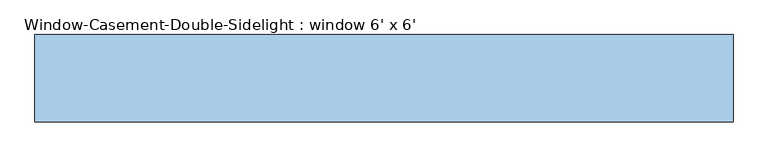
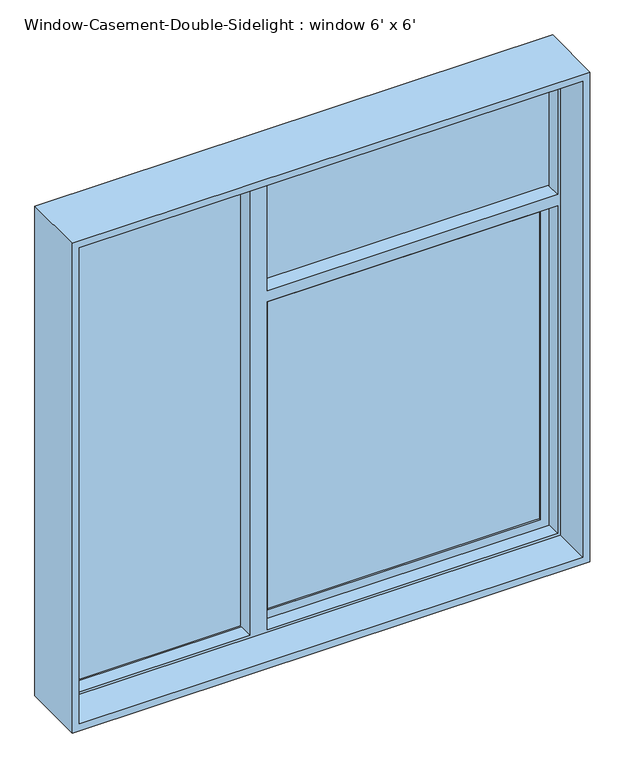
"""IFC4 building model written with IfcOpenShell, lengths in millimetres: window geometry, Window-Casement-Double-Sidelight : window 6' x 6'."""

from ifc_helpers import new_model, si_unit, frame, origin, place, context, project, spatial, polyline, outline, extrude, faceted_brep, source, transform, mapped, element, save


def window_casement_double_sidelight_window_6_x_6_6a7c62ef(model_context):
    return source(origin(), model_context, "Body", "SolidModel", [
        extrude(outline(polyline([(847.1296875, 98.425), (-115.6096875, 98.425), (-115.6096875, 111.125), (847.1296875, 111.125), (847.1296875, 98.425)])), frame((0.0, 0.0, 981.6703125), z_axis=(0.0, 0.0, 1.0), x_axis=(1.0, 0.0, 0.0)), (0.0, 0.0, 1.0), 1150.0842187),
        extrude(outline(polyline([(847.1296875, 85.725), (847.1296875, 79.375), (-115.6096875, 79.375), (-115.6096875, 85.725), (847.1296875, 85.725)])), frame((0.0, 0.0, 981.6703125), z_axis=(0.0, 0.0, 1.0), x_axis=(1.0, 0.0, 0.0)), (0.0, 0.0, 1.0), 1150.0842187),
        extrude(outline(polyline([(-208.28, 98.425), (-208.28, 92.075), (-889.0, 92.075), (-889.0, 98.425), (-208.28, 98.425)])), frame((0.0, 0.0, 949.9203125), z_axis=(0.0, 0.0, 1.0), x_axis=(1.0, 0.0, 0.0)), (0.0, 0.0, 1.0), 1767.8796875),
        extrude(outline(polyline([(-208.28, 85.725), (-208.28, 79.375), (-889.0, 79.375), (-889.0, 85.725), (-208.28, 85.725)])), frame((0.0, 0.0, 949.9203125), z_axis=(0.0, 0.0, 1.0), x_axis=(1.0, 0.0, 0.0)), (0.0, 0.0, 1.0), 1767.8796875),
        extrude(outline(polyline([(889.0, 85.725), (889.0, 79.375), (-157.48, 79.375), (-157.48, 85.725), (889.0, 85.725)])), frame((0.0, 0.0, 2215.4951563), z_axis=(0.0, 0.0, 1.0), x_axis=(1.0, 0.0, 0.0)), (0.0, 0.0, 1.0), 502.3048438),
        extrude(outline(polyline([(889.0, 98.425), (889.0, 92.075), (-157.48, 92.075), (-157.48, 98.425), (889.0, 98.425)])), frame((0.0, 0.0, 2215.4951563), z_axis=(0.0, 0.0, 1.0), x_axis=(1.0, 0.0, 0.0)), (0.0, 0.0, 1.0), 502.3048438),
        faceted_brep([(-889.0, 73.025, 2717.8), (-889.0, 114.3, 2717.8), (889.0, 114.3, 2717.8), (889.0, 73.025, 2717.8), (-157.48, 73.025, 2717.8), (-157.48, 111.125, 2717.8), (-208.28, 111.125, 2717.8), (-208.28, 73.025, 2717.8), (-878.8796875, 22.225, 2707.6796875), (-878.8796875, 73.025, 2707.6796875), (-208.28, 73.025, 2707.6796875), (-208.28, 22.225, 2707.6796875), (878.8796875, 73.025, 2707.6796875), (878.8796875, 22.225, 2707.6796875), (-147.3596875, 22.225, 2707.6796875), (-147.3596875, 73.025, 2707.6796875), (-889.0, -114.3, 2717.8), (-889.0, 22.225, 2717.8), (889.0, 22.225, 2717.8), (889.0, -114.3, 2717.8), (-914.4, 114.3, 2743.2), (-914.4, -114.3, 2743.2), (914.4, -114.3, 2743.2), (914.4, 114.3, 2743.2), (889.0, 114.3, 939.8), (889.0, 73.025, 939.8), (889.0, 73.025, 2173.6248438), (889.0, 111.125, 2173.6248438), (889.0, 111.125, 2215.4951563), (889.0, 73.025, 2215.4951563), (878.8796875, 73.025, 2215.4951563), (878.8796875, 22.225, 2215.4951563), (878.8796875, 73.025, 949.9203125), (878.8796875, 22.225, 949.9203125), (878.8796875, 22.225, 2173.6248438), (878.8796875, 73.025, 2173.6248438), (889.0, 22.225, 939.8), (889.0, -114.3, 939.8), (914.4, -114.3, 914.4), (914.4, 114.3, 914.4), (-889.0, 114.3, 939.8), (-889.0, 73.025, 939.8), (-208.28, 73.025, 939.8), (-208.28, 111.125, 939.8), (-157.48, 111.125, 939.8), (-157.48, 73.025, 939.8), (-147.3596875, 73.025, 949.9203125), (-147.3596875, 22.225, 949.9203125), (-878.8796875, 73.025, 949.9203125), (-878.8796875, 22.225, 949.9203125), (-208.28, 22.225, 949.9203125), (-208.28, 73.025, 949.9203125), (-889.0, 22.225, 939.8), (-889.0, -114.3, 939.8), (-914.4, -114.3, 914.4), (-914.4, 114.3, 914.4), (-147.3596875, 73.025, 2215.4951563), (-157.48, 73.025, 2215.4951563), (-157.48, 73.025, 2173.6248438), (-147.3596875, 73.025, 2173.6248438), (-147.3596875, 22.225, 2215.4951563), (-147.3596875, 22.225, 2173.6248438), (-157.48, 111.125, 2215.4951563), (-157.48, 111.125, 2173.6248438)], [[[0, 1, 2, 3, 4, 5, 6, 7]], [[8, 9, 10, 11]], [[12, 13, 14, 15]], [[16, 17, 18, 19]], [[20, 21, 22, 23]], [[3, 2, 24, 25, 26, 27, 28, 29]], [[13, 12, 30, 31]], [[32, 33, 34, 35]], [[19, 18, 36, 37]], [[23, 22, 38, 39]], [[25, 24, 40, 41, 42, 43, 44, 45]], [[33, 32, 46, 47]], [[48, 49, 50, 51]], [[37, 36, 52, 53]], [[39, 38, 54, 55]], [[1, 0, 41, 40]], [[12, 15, 56, 57, 4, 3, 29, 30]], [[46, 32, 35, 26, 25, 45, 58, 59]], [[41, 0, 7, 10, 9, 48, 51, 42]], [[9, 8, 49, 48]], [[17, 52, 36, 18], [13, 31, 60, 14], [33, 47, 61, 34], [49, 8, 11, 50]], [[17, 16, 53, 52]], [[22, 21, 54, 38], [16, 19, 37, 53]], [[21, 20, 55, 54]], [[20, 23, 39, 55], [2, 1, 40, 24]], [[43, 6, 5, 62, 28, 27, 63, 44]], [[6, 43, 42, 51, 50, 11, 10, 7]], [[15, 14, 60, 56]], [[47, 46, 59, 61]], [[5, 4, 57, 62]], [[45, 44, 63, 58]], [[63, 27, 26, 35, 34, 61, 59, 58]], [[28, 62, 57, 56, 60, 31, 30, 29]]]),
        extrude(outline(polyline([(2173.6248438, 889.0), (2173.6248438, -157.48), (939.8, -157.48), (939.8, 889.0), (2173.6248438, 889.0)]), holes=[polyline([(981.6703125, 847.1296875), (981.6703125, -115.6096875), (2131.7545313, -115.6096875), (2131.7545313, 847.1296875), (981.6703125, 847.1296875)])]), frame((0.0, 73.025, 0.0), z_axis=(0.0, 1.0, 0.0), x_axis=(0.0, 0.0, 1.0)), (0.0, 0.0, 1.0), 31.75),
    ])


if __name__ == "__main__":
    model = new_model("IFC4")
    model_context = context("Model", 3, world=origin())
    ifc_project = project(units=[si_unit("LENGTHUNIT", "METRE", prefix="MILLI")], contexts=[model_context])
    site = spatial("IfcSite", under=ifc_project)
    building = spatial("IfcBuilding", under=site)
    placement = place(None, origin())
    window_casement_double_sidelight_window_6_x_6_shape = window_casement_double_sidelight_window_6_x_6_6a7c62ef(model_context)
    element("IfcWindow", 1, ObjectType="Window-Casement-Double-Sidelight : window 6' x 6'", at=placement, inside=building, context=model_context, shape_type="MappedRepresentation", body=[
        mapped(window_casement_double_sidelight_window_6_x_6_shape, transform((0.0, 0.0, 0.0), x_axis=(1.0, 0.0, 0.0), y_axis=(0.0, 1.0, 0.0), z_axis=(0.0, 0.0, 1.0))),
    ])
    save(model, "model.ifc")

# Revit data of these elements
# Type "Window-Casement-Double-Sidelight : window 6' x 6'"
#   Type Mark = "23"
#   Fire Rating = "0.5h"
#   Assembly Code = "B2020100"
#   Analytic Construction = "Double glazing - domestic"
#   Window Inset [instance default] = 0' - 0 5/8"
#   Wall Thickness [instance default] = 0' - 6"
#   Visual Light Transmittance = 0.81
#   Transom Height Ratio = 0.3
#   Transom Height = 1' - 9.6"
#   Thermal Resistance (R) = 1.8146 (h·ft²·°F)/BTU
#   Solar Heat Gain Coefficient = 0.76
#   Side Width = 2' - 4.8"
#   Rough Width = 6' - 0 1/2"
#   Rough Height = 6' - 0 1/2"
#   Opening Window Width = 3' - 7.2"
#   Opening Window Height = 4' - 2.4"
#   Heat Transfer Coefficient (U) = 0.5511 BTU/(h·ft²·°F)
#   Height = 6' - 0"
#   Frame Gap 3 [instance default] = 0' - 1 83/128"
#   Frame Gap 2 [instance default] = 0' - 0 5/8"
#   Frame Gap 1 = 0' - 1 51/128"
#   Default Sill Height = 3' - 0"
#   Width = 6' - 0"
#   Frame Material = Metal - Aluminum
#   Glass Panel Material = Glass
#   Wall Closure = (empty or 0)
# Element 1 (IfcWindow, "Window-Casement-Double-Sidelight : window 6' x 6'")
#   Wall Thickness = 0' - 9"
#   Materials on its faces: "Metal - Aluminum", "Glass"
# Materials
#   "Metal - Aluminum": class "Metal", colour RGB 247 247 247, transparency 0
#   "Glass": class "Glass", colour RGB 0 128 192, transparency 0.75, Description = "Soda Lime Glass", Cost = 0
